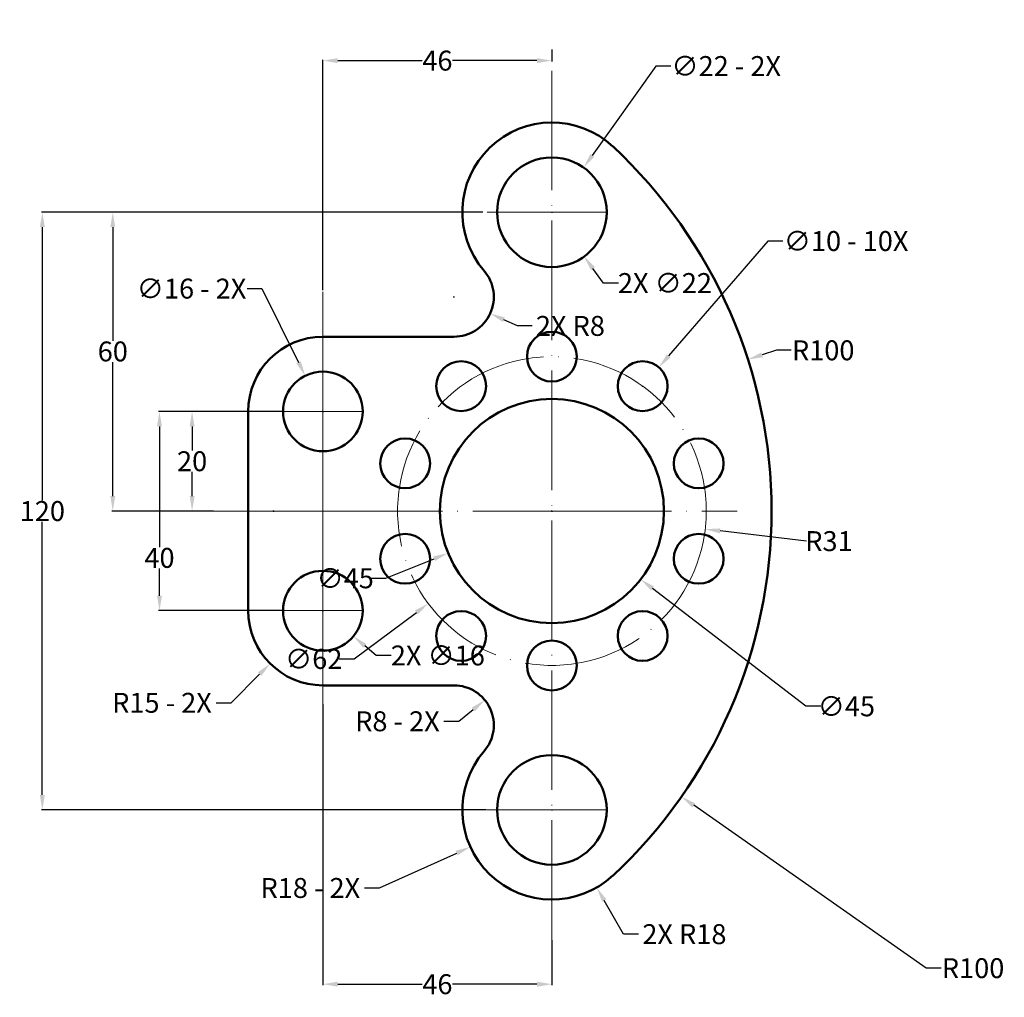
# Model space of a CAD drawing. Units: inches. Extents: x 498 to 696, y 198 to 394.
import ezdxf

# ---------------------------------------------------------------- set-up
doc = ezdxf.new("R2010")
doc.units = ezdxf.units.IN
doc.header["$MEASUREMENT"] = 0
doc.linetypes.add('ACAD_ISO04W100', pattern=[30, 24, -3, 0, -3])
for name, color, linetype, lineweight in [('M-CNTR', 4, 'ACAD_ISO04W100', 18), ('M-DIMS', 2, 'Continuous', 25), ('M-OUTL', 7, 'Continuous', 50)]:
    doc.layers.add(name, color=color, linetype=linetype, lineweight=lineweight)
doc.styles.get("Standard").update_dxf_attribs({"font": 'arial.ttf'})
doc.dimstyles.get("Standard").update_dxf_attribs({"dimtxt": 4, "dimasz": 3, "dimexe": 0.18, "dimexo": 0.0625, "dimgap": 0.09, "dimtad": 0, "dimtih": 1, "dimtoh": 1, "dimdec": 0, "dimzin": 0, "dimdsep": 46, "dimtxsty": 'Standard', "dimcen": 0.09, "dimclrd": 1, "dimclre": 1, "dimadec": 0, "dimazin": 0, "dimtfac": 1, "dimtdec": 0, "dimtofl": 0, "dimtmove": 0, "dimatfit": 3, "dimfxl": 1, "dimtolj": 1, "dimtzin": 0, "dimarcsym": 0})

# ---------------------------------------------------------------- blocks, each defined once
blk = doc.blocks.new('*U1')
blk.add_circle((0, 0), 5)
blk = doc.blocks.new('*U2')
at = {"layer": 'M-OUTL', "color": 0, "linetype": 'ByBlock', "lineweight": -2, "transparency": 16777216}
blk.add_blockref('*U1', (604.82, 326.53), dxfattribs=at)
for p, rotation in [((586.6, 320.6), 35.99999999999999), ((623.04, 320.6), 324), ((575.34, 305.1), 72), ((634.3, 305.1), 288), ((575.34, 285.95), 108), ((634.3, 285.95), 252), ((586.6, 270.45), 144), ((623.04, 270.45), 216), ((604.82, 264.53), 180)]:
    blk.add_blockref('*U1', p, dxfattribs=dict(at, rotation=rotation))
blk = doc.blocks.new('*D3')
at = {"layer": 'Defpoints', "color": 0, "transparency": 16777216}
for p in [(591.02, 355.53), (502.47, 235.53), (591.74, 235.53)]:
    blk.add_point(p, dxfattribs=at)
at = {"layer": 'M-DIMS', "color": 0, "lineweight": -2, "transparency": 16777216}
for p, q in [((590.96, 355.53), (502.29, 355.53)), ((502.47, 352.53), (502.47, 297.66)), ((502.47, 238.53), (502.47, 293.39)), ((591.68, 235.53), (502.29, 235.53))]:
    blk.add_line(p, q, dxfattribs=at)
at = {"layer": 'M-DIMS', "color": 0, "transparency": 16777216}
for points in [[(501.97, 352.53), (502.97, 352.53), (502.47, 355.53)], [(501.97, 238.53), (502.97, 238.53), (502.47, 235.53)]]:
    blk.add_solid(points, dxfattribs=at)
at = {"layer": 'M-DIMS', "color": 0, "transparency": 16777216, "insert": (502.47, 295.53), "char_height": 4, "attachment_point": 5}
blk.add_mtext('\\A1;120', dxfattribs=at)
blk = doc.blocks.new('*D4')
at = {"layer": 'Defpoints', "color": 0, "transparency": 16777216}
for p in [(591.02, 355.53), (516.62, 295.53), (536.94, 295.53)]:
    blk.add_point(p, dxfattribs=at)
at = {"layer": 'M-DIMS', "color": 0, "lineweight": -2, "transparency": 16777216}
for p, q in [((590.96, 355.53), (516.44, 355.53)), ((516.62, 352.53), (516.62, 329.7)), ((516.62, 298.53), (516.62, 325.44)), ((536.88, 295.53), (516.44, 295.53))]:
    blk.add_line(p, q, dxfattribs=at)
at = {"layer": 'M-DIMS', "color": 0, "transparency": 16777216}
for points in [[(516.12, 352.53), (517.12, 352.53), (516.62, 355.53)], [(516.12, 298.53), (517.12, 298.53), (516.62, 295.53)]]:
    blk.add_solid(points, dxfattribs=at)
at = {"layer": 'M-DIMS', "color": 0, "transparency": 16777216, "insert": (516.62, 327.57), "char_height": 4, "attachment_point": 5}
blk.add_mtext('\\A1;60', dxfattribs=at)
blk = doc.blocks.new('*D5')
at = {"layer": 'Defpoints', "color": 0, "transparency": 16777216}
for p in [(555.26, 322.69), (562.38, 308.36)]:
    blk.add_point(p, dxfattribs=at)
at = {"layer": 'M-DIMS', "color": 0, "lineweight": -2, "transparency": 16777216}
for p, q in [((543.58, 340.19), (546.58, 340.19)), ((546.58, 340.19), (553.93, 325.38)), ((558.73, 315.53), (558.91, 315.53)), ((558.82, 315.44), (558.82, 315.62))]:
    blk.add_line(p, q, dxfattribs=at)
at = {"layer": 'M-DIMS', "color": 0, "transparency": 16777216}
blk.add_solid([(554.38, 325.6), (553.48, 325.16), (555.26, 322.69)], dxfattribs=at)
at = {"layer": 'M-DIMS', "color": 0, "transparency": 16777216, "insert": (532.44, 340.19), "char_height": 4, "attachment_point": 5}
blk.add_mtext('\\A1;∅16 - 2X', dxfattribs=at)
blk = doc.blocks.new('*D6')
at = {"layer": 'Defpoints', "color": 0, "transparency": 16777216}
for p in [(550.82, 315.53), (532.55, 295.53), (536.94, 295.53)]:
    blk.add_point(p, dxfattribs=at)
at = {"layer": 'M-DIMS', "color": 0, "lineweight": -2, "transparency": 16777216}
for p, q in [((550.76, 315.53), (532.37, 315.53)), ((532.55, 312.53), (532.55, 307.66)), ((532.55, 298.53), (532.55, 303.39)), ((536.88, 295.53), (532.37, 295.53))]:
    blk.add_line(p, q, dxfattribs=at)
at = {"layer": 'M-DIMS', "color": 0, "transparency": 16777216}
for points in [[(532.05, 312.53), (533.05, 312.53), (532.55, 315.53)], [(532.05, 298.53), (533.05, 298.53), (532.55, 295.53)]]:
    blk.add_solid(points, dxfattribs=at)
at = {"layer": 'M-DIMS', "color": 0, "transparency": 16777216, "insert": (532.55, 305.53), "char_height": 4, "attachment_point": 5}
blk.add_mtext('\\A1;20', dxfattribs=at)
blk = doc.blocks.new('*D7')
at = {"layer": 'Defpoints', "color": 0, "transparency": 16777216}
for p in [(550.82, 315.53), (526, 275.53), (550.82, 275.53)]:
    blk.add_point(p, dxfattribs=at)
at = {"layer": 'M-DIMS', "color": 0, "lineweight": -2, "transparency": 16777216}
for p, q in [((550.76, 315.53), (525.82, 315.53)), ((526, 312.53), (526, 288.25)), ((526, 278.53), (526, 283.99)), ((550.76, 275.53), (525.82, 275.53))]:
    blk.add_line(p, q, dxfattribs=at)
at = {"layer": 'M-DIMS', "color": 0, "transparency": 16777216}
for points in [[(525.5, 312.53), (526.5, 312.53), (526, 315.53)], [(525.5, 278.53), (526.5, 278.53), (526, 275.53)]]:
    blk.add_solid(points, dxfattribs=at)
at = {"layer": 'M-DIMS', "color": 0, "transparency": 16777216, "insert": (526, 286.12), "char_height": 4, "attachment_point": 5}
blk.add_mtext('\\A1;40', dxfattribs=at)
blk = doc.blocks.new('*D8')
at = {"layer": 'Defpoints', "color": 0, "transparency": 16777216}
for p in [(558.82, 275.53), (548.23, 264.9)]:
    blk.add_point(p, dxfattribs=at)
at = {"layer": 'M-DIMS', "color": 0, "lineweight": -2, "transparency": 16777216}
for p, q in [((558.73, 275.53), (558.91, 275.53)), ((558.82, 275.44), (558.82, 275.62)), ((540.38, 257.03), (546.11, 262.78)), ((537.38, 257.03), (540.38, 257.03))]:
    blk.add_line(p, q, dxfattribs=at)
at = {"layer": 'M-DIMS', "color": 0, "transparency": 16777216}
blk.add_solid([(545.76, 263.13), (546.46, 262.43), (548.23, 264.9)], dxfattribs=at)
at = {"layer": 'M-DIMS', "color": 0, "transparency": 16777216, "insert": (526.5, 257.03), "char_height": 4, "attachment_point": 5}
blk.add_mtext('\\A1;R15 - 2X', dxfattribs=at)
blk = doc.blocks.new('*D9')
at = {"layer": 'Defpoints', "color": 0, "transparency": 16777216}
for p in [(591.35, 257.58), (585.15, 252.53)]:
    blk.add_point(p, dxfattribs=at)
at = {"layer": 'M-DIMS', "color": 0, "lineweight": -2, "transparency": 16777216}
for p, q in [((586.12, 253.32), (589.02, 255.69)), ((583.12, 253.32), (586.12, 253.32))]:
    blk.add_line(p, q, dxfattribs=at)
at = {"layer": 'M-DIMS', "color": 0, "transparency": 16777216}
blk.add_solid([(588.71, 256.07), (589.34, 255.3), (591.35, 257.58)], dxfattribs=at)
at = {"layer": 'M-DIMS', "color": 0, "transparency": 16777216, "insert": (573.79, 253.32), "char_height": 4, "attachment_point": 5}
blk.add_mtext('\\A1;R8 - 2X', dxfattribs=at)
blk = doc.blocks.new('*D10')
at = {"layer": 'Defpoints', "color": 0, "transparency": 16777216}
for p in [(604.82, 235.53), (588.42, 228.1)]:
    blk.add_point(p, dxfattribs=at)
at = {"layer": 'M-DIMS', "color": 0, "lineweight": -2, "transparency": 16777216}
for p, q in [((604.73, 235.53), (604.91, 235.53)), ((604.82, 235.44), (604.82, 235.62)), ((570.18, 219.85), (585.69, 226.87)), ((567.18, 219.85), (570.18, 219.85))]:
    blk.add_line(p, q, dxfattribs=at)
at = {"layer": 'M-DIMS', "color": 0, "transparency": 16777216}
blk.add_solid([(585.48, 227.32), (585.9, 226.41), (588.42, 228.1)], dxfattribs=at)
at = {"layer": 'M-DIMS', "color": 0, "transparency": 16777216, "insert": (556.3, 219.85), "char_height": 4, "attachment_point": 5}
blk.add_mtext('\\A1;R18 - 2X', dxfattribs=at)
blk = doc.blocks.new('*D11')
at = {"layer": 'Defpoints', "color": 0, "transparency": 16777216}
for p in [(558.82, 256.82), (604.82, 209.44), (604.82, 200.53)]:
    blk.add_point(p, dxfattribs=at)
at = {"layer": 'M-DIMS', "color": 0, "lineweight": -2, "transparency": 16777216}
for p, q in [((558.82, 256.75), (558.82, 200.35)), ((604.82, 209.37), (604.82, 200.35)), ((561.82, 200.53), (578.79, 200.53)), ((601.82, 200.53), (584.85, 200.53))]:
    blk.add_line(p, q, dxfattribs=at)
at = {"layer": 'M-DIMS', "color": 0, "transparency": 16777216}
for points in [[(561.82, 201.03), (561.82, 200.03), (558.82, 200.53)], [(601.82, 201.03), (601.82, 200.03), (604.82, 200.53)]]:
    blk.add_solid(points, dxfattribs=at)
at = {"layer": 'M-DIMS', "color": 0, "transparency": 16777216, "insert": (581.82, 200.53), "char_height": 4, "attachment_point": 5}
blk.add_mtext('\\A1;46', dxfattribs=at)
blk = doc.blocks.new('*D12')
at = {"layer": 'Defpoints', "color": 0, "transparency": 16777216}
for p in [(586.98, 309.24), (622.66, 281.81)]:
    blk.add_point(p, dxfattribs=at)
at = {"layer": 'M-DIMS', "color": 0, "lineweight": -2, "transparency": 16777216}
for p, q in [((604.73, 295.53), (604.91, 295.53)), ((604.82, 295.44), (604.82, 295.62)), ((655.81, 256.32), (625.04, 279.98)), ((658.81, 256.32), (655.81, 256.32))]:
    blk.add_line(p, q, dxfattribs=at)
at = {"layer": 'M-DIMS', "color": 0, "transparency": 16777216}
blk.add_solid([(625.34, 280.38), (624.73, 279.59), (622.66, 281.81)], dxfattribs=at)
at = {"layer": 'M-DIMS', "color": 0, "transparency": 16777216, "insert": (663.96, 256.32), "char_height": 4, "attachment_point": 5}
blk.add_mtext('\\A1;∅45', dxfattribs=at)
blk = doc.blocks.new('*D13')
at = {"layer": 'Defpoints', "color": 0, "transparency": 16777216}
for p in [(604.82, 295.53), (635.61, 291.89)]:
    blk.add_point(p, dxfattribs=at)
at = {"layer": 'M-DIMS', "color": 0, "lineweight": -2, "transparency": 16777216}
for p, q in [((604.73, 295.53), (604.91, 295.53)), ((604.82, 295.44), (604.82, 295.62)), ((655.98, 289.49), (638.59, 291.54))]:
    blk.add_line(p, q, dxfattribs=at)
at = {"layer": 'M-DIMS', "color": 0, "transparency": 16777216}
blk.add_solid([(638.64, 292.04), (638.53, 291.04), (635.61, 291.89)], dxfattribs=at)
at = {"layer": 'M-DIMS', "color": 0, "transparency": 16777216, "insert": (660.46, 289.49), "char_height": 4, "attachment_point": 5}
blk.add_mtext('\\A1;R31', dxfattribs=at)
blk = doc.blocks.new('*D14')
at = {"layer": 'Defpoints', "color": 0, "transparency": 16777216}
for p in [(644.18, 325.97), (548.93, 295.53)]:
    blk.add_point(p, dxfattribs=at)
at = {"layer": 'M-DIMS', "color": 0, "lineweight": -2, "transparency": 16777216}
for p, q in [((649.9, 327.8), (647.04, 326.89)), ((652.9, 327.8), (649.9, 327.8)), ((548.84, 295.53), (549.02, 295.53)), ((548.93, 295.44), (548.93, 295.62))]:
    blk.add_line(p, q, dxfattribs=at)
at = {"layer": 'M-DIMS', "color": 0, "transparency": 16777216}
blk.add_solid([(646.89, 327.36), (647.19, 326.41), (644.18, 325.97)], dxfattribs=at)
at = {"layer": 'M-DIMS', "color": 0, "transparency": 16777216, "insert": (659.31, 327.8), "char_height": 4, "attachment_point": 5}
blk.add_mtext('\\A1;R100', dxfattribs=at)
blk = doc.blocks.new('*D15')
at = {"layer": 'Defpoints', "color": 0, "transparency": 16777216}
for p in [(626.31, 324.39), (619.77, 316.82)]:
    blk.add_point(p, dxfattribs=at)
at = {"layer": 'M-DIMS', "color": 0, "lineweight": -2, "transparency": 16777216}
for p, q in [((648.21, 349.74), (628.27, 326.66)), ((651.21, 349.74), (648.21, 349.74)), ((622.95, 320.6), (623.13, 320.6)), ((623.04, 320.51), (623.04, 320.69))]:
    blk.add_line(p, q, dxfattribs=at)
at = {"layer": 'M-DIMS', "color": 0, "transparency": 16777216}
blk.add_solid([(627.89, 326.99), (628.65, 326.33), (626.31, 324.39)], dxfattribs=at)
at = {"layer": 'M-DIMS', "color": 0, "transparency": 16777216, "insert": (663.91, 349.74), "char_height": 4, "attachment_point": 5}
blk.add_mtext('\\A1;∅10 - 10X', dxfattribs=at)
blk = doc.blocks.new('*D16')
at = {"layer": 'Defpoints', "color": 0, "transparency": 16777216}
for p in [(611.2, 364.49), (598.45, 346.56)]:
    blk.add_point(p, dxfattribs=at)
at = {"layer": 'M-DIMS', "color": 0, "lineweight": -2, "transparency": 16777216}
for p, q in [((625.69, 384.87), (612.93, 366.93)), ((628.69, 384.87), (625.69, 384.87)), ((604.73, 355.53), (604.91, 355.53)), ((604.82, 355.44), (604.82, 355.62))]:
    blk.add_line(p, q, dxfattribs=at)
at = {"layer": 'M-DIMS', "color": 0, "transparency": 16777216}
blk.add_solid([(612.53, 367.22), (613.34, 366.64), (611.2, 364.49)], dxfattribs=at)
at = {"layer": 'M-DIMS', "color": 0, "transparency": 16777216, "insert": (639.83, 384.87), "char_height": 4, "attachment_point": 5}
blk.add_mtext('\\A1;∅22 - 2X', dxfattribs=at)
blk = doc.blocks.new('*D17')
at = {"layer": 'Defpoints', "color": 0, "transparency": 16777216}
for p in [(604.82, 388.24), (604.82, 385.96), (558.82, 339.8)]:
    blk.add_point(p, dxfattribs=at)
at = {"layer": 'M-DIMS', "color": 0, "lineweight": -2, "transparency": 16777216}
for p, q in [((604.82, 388.17), (604.82, 385.78)), ((558.82, 339.86), (558.82, 386.14)), ((561.82, 385.96), (578.79, 385.96)), ((601.82, 385.96), (584.85, 385.96))]:
    blk.add_line(p, q, dxfattribs=at)
at = {"layer": 'M-DIMS', "color": 0, "transparency": 16777216}
for points in [[(561.82, 386.46), (561.82, 385.46), (558.82, 385.96)], [(601.82, 386.46), (601.82, 385.46), (604.82, 385.96)]]:
    blk.add_solid(points, dxfattribs=at)
at = {"layer": 'M-DIMS', "color": 0, "transparency": 16777216, "insert": (581.82, 385.96), "char_height": 4, "attachment_point": 5}
blk.add_mtext('\\A1;46', dxfattribs=at)
blk = doc.blocks.new('HOLE-MOUNT-D16')
blk.add_circle((8, 8), 8)
blk = doc.blocks.new('HOLE-EAR-D22')
blk.add_circle((11, 11), 11)
blk = doc.blocks.new('*D20')
at = {"layer": 'Defpoints', "color": 0, "transparency": 16777216}
for p in [(548.93, 295.53), (630.84, 238.17)]:
    blk.add_point(p, dxfattribs=at)
at = {"layer": 'M-DIMS', "color": 1, "lineweight": -2, "transparency": 16777216}
for p, q in [((548.84, 295.53), (549.02, 295.53)), ((548.93, 295.44), (548.93, 295.62)), ((679.99, 203.75), (633.3, 236.45)), ((682.99, 203.75), (679.99, 203.75))]:
    blk.add_line(p, q, dxfattribs=at)
at = {"layer": 'M-DIMS', "color": 1, "transparency": 16777216}
blk.add_solid([(633.59, 236.86), (633.01, 236.04), (630.84, 238.17)], dxfattribs=at)
at = {"layer": 'M-DIMS', "color": 0, "transparency": 16777216, "insert": (689.41, 203.75), "char_height": 4, "attachment_point": 5}
blk.add_mtext('\\A1;R100', dxfattribs=at)
blk = doc.blocks.new('*D21')
at = {"layer": 'Defpoints', "color": 0, "transparency": 16777216}
for p in [(625.68, 303.96), (583.96, 287.09)]:
    blk.add_point(p, dxfattribs=at)
at = {"layer": 'M-DIMS', "color": 1, "lineweight": -2, "transparency": 16777216}
for p, q in [((604.73, 295.53), (604.91, 295.53)), ((604.82, 295.44), (604.82, 295.62)), ((571.45, 282.02), (581.18, 285.96)), ((568.45, 282.02), (571.45, 282.02))]:
    blk.add_line(p, q, dxfattribs=at)
at = {"layer": 'M-DIMS', "color": 1, "transparency": 16777216}
blk.add_solid([(580.99, 286.42), (581.37, 285.5), (583.96, 287.09)], dxfattribs=at)
at = {"layer": 'M-DIMS', "color": 0, "transparency": 16777216, "insert": (563.3, 282.02), "char_height": 4, "attachment_point": 5}
blk.add_mtext('\\A1;∅45', dxfattribs=at)
blk = doc.blocks.new('*D22')
at = {"layer": 'Defpoints', "color": 0, "transparency": 16777216}
for p in [(629.65, 314.09), (579.99, 276.96)]:
    blk.add_point(p, dxfattribs=at)
at = {"layer": 'M-DIMS', "color": 1, "lineweight": -2, "transparency": 16777216}
for p, q in [((604.73, 295.53), (604.91, 295.53)), ((604.82, 295.44), (604.82, 295.62)), ((565.09, 265.83), (577.59, 275.17)), ((562.09, 265.83), (565.09, 265.83))]:
    blk.add_line(p, q, dxfattribs=at)
at = {"layer": 'M-DIMS', "color": 1, "transparency": 16777216}
blk.add_solid([(577.29, 275.57), (577.89, 274.77), (579.99, 276.96)], dxfattribs=at)
at = {"layer": 'M-DIMS', "color": 0, "transparency": 16777216, "insert": (556.98, 265.83), "char_height": 4, "attachment_point": 5}
blk.add_mtext('\\A1;∅62', dxfattribs=at)
blk = doc.blocks.new('*D23')
at = {"layer": 'Defpoints', "color": 0, "transparency": 16777216}
for p in [(604.82, 235.53), (613.82, 219.94)]:
    blk.add_point(p, dxfattribs=at)
at = {"layer": 'M-DIMS', "color": 1, "lineweight": -2, "transparency": 16777216}
for p, q in [((604.73, 235.53), (604.91, 235.53)), ((604.82, 235.44), (604.82, 235.62)), ((619.22, 210.58), (615.32, 217.34)), ((622.22, 210.58), (619.22, 210.58))]:
    blk.add_line(p, q, dxfattribs=at)
at = {"layer": 'M-DIMS', "color": 1, "transparency": 16777216}
blk.add_solid([(615.75, 217.59), (614.89, 217.09), (613.82, 219.94)], dxfattribs=at)
at = {"layer": 'M-DIMS', "color": 0, "transparency": 16777216, "insert": (631.43, 210.58), "char_height": 4, "attachment_point": 5}
blk.add_mtext('\\A1;2X R18', dxfattribs=at)
blk = doc.blocks.new('*D24')
at = {"layer": 'Defpoints', "color": 0, "transparency": 16777216}
for p in [(585.15, 338.53), (592.42, 335.2)]:
    blk.add_point(p, dxfattribs=at)
at = {"layer": 'M-DIMS', "color": 1, "lineweight": -2, "transparency": 16777216}
for p, q in [((585.06, 338.53), (585.24, 338.53)), ((585.15, 338.44), (585.15, 338.62)), ((597.88, 332.7), (595.15, 333.95)), ((600.88, 332.7), (597.88, 332.7))]:
    blk.add_line(p, q, dxfattribs=at)
at = {"layer": 'M-DIMS', "color": 1, "transparency": 16777216}
blk.add_solid([(595.36, 334.4), (594.94, 333.49), (592.42, 335.2)], dxfattribs=at)
at = {"layer": 'M-DIMS', "color": 0, "transparency": 16777216, "insert": (608.53, 332.7), "char_height": 4, "attachment_point": 5}
blk.add_mtext('\\A1;2X R8', dxfattribs=at)
blk = doc.blocks.new('*D25')
at = {"layer": 'Defpoints', "color": 0, "transparency": 16777216}
for p in [(598.34, 364.42), (611.3, 346.63)]:
    blk.add_point(p, dxfattribs=at)
at = {"layer": 'M-DIMS', "color": 1, "lineweight": -2, "transparency": 16777216}
for p, q in [((604.73, 355.53), (604.91, 355.53)), ((604.82, 355.44), (604.82, 355.62)), ((615.18, 341.3), (613.06, 344.21)), ((618.18, 341.3), (615.18, 341.3))]:
    blk.add_line(p, q, dxfattribs=at)
at = {"layer": 'M-DIMS', "color": 1, "transparency": 16777216}
blk.add_solid([(613.47, 344.5), (612.66, 343.91), (611.3, 346.63)], dxfattribs=at)
at = {"layer": 'M-DIMS', "color": 0, "transparency": 16777216, "insert": (627.52, 341.3), "char_height": 4, "attachment_point": 5}
blk.add_mtext('\\A1;2X ∅22', dxfattribs=at)
blk = doc.blocks.new('*D26')
at = {"layer": 'Defpoints', "color": 0, "transparency": 16777216}
for p in [(552.69, 280.66), (564.95, 270.39)]:
    blk.add_point(p, dxfattribs=at)
at = {"layer": 'M-DIMS', "color": 1, "lineweight": -2, "transparency": 16777216}
for p, q in [((558.73, 275.53), (558.91, 275.53)), ((558.82, 275.44), (558.82, 275.62)), ((569.55, 266.53), (567.25, 268.46)), ((572.55, 266.53), (569.55, 266.53))]:
    blk.add_line(p, q, dxfattribs=at)
at = {"layer": 'M-DIMS', "color": 1, "transparency": 16777216}
blk.add_solid([(567.57, 268.84), (566.93, 268.08), (564.95, 270.39)], dxfattribs=at)
at = {"layer": 'M-DIMS', "color": 0, "transparency": 16777216, "insert": (581.91, 266.53), "char_height": 4, "attachment_point": 5}
blk.add_mtext('\\A1;2X ∅16', dxfattribs=at)

msp = doc.modelspace()

# ---------------------------------------------------------------- linework, layer by layer
at = {"layer": 'M-CNTR'}
for p, q in [((604.82, 209.44), (604.82, 388.24)), ((615.82, 355.53), (591.02, 355.53)), ((566.82, 315.53), (550.82, 315.53)), ((566.82, 275.53), (550.82, 275.53)), ((615.82, 235.53), (591.74, 235.53))]:
    msp.add_line(p, q, dxfattribs=at)
for points in [[(558.82, 256.82), (558.82, 275.53), (558.82, 295.53), (558.82, 315.53), (558.82, 339.8)], [(536.94, 295.53), (558.82, 295.53), (604.82, 295.53), (642, 295.53)]]:
    msp.add_lwpolyline(points, dxfattribs=at)
msp.add_circle((604.82, 295.53), 31, dxfattribs=at)
at = {"layer": 'M-OUTL'}
for p, q in [((558.82, 330.53), (585.15, 330.53)), ((543.82, 315.53), (543.82, 275.53)), ((558.82, 260.53), (585.15, 260.53))]:
    msp.add_line(p, q, dxfattribs=at)
msp.add_circle((604.82, 295.53), 22.5, dxfattribs=at)
for centre, radius, start, end in [((604.82, 355.53), 18, 47.0297, 220.8322), ((548.93, 295.53), 100, 312.9703, 47.0297), ((585.15, 338.53), 8, 270, 40.8322), ((558.82, 315.53), 15, 90, 180), ((558.82, 275.53), 15, 180, 270), ((585.15, 252.53), 8, 319.1678, 90), ((604.82, 235.53), 18, 139.1678, 312.9703)]:
    msp.add_arc(centre, radius, start, end, dxfattribs=at)

# ---------------------------------------------------------------- block references
for name, p in [('HOLE-EAR-D22', (593.82, 344.52)), ('*U2', (0, 0)), ('HOLE-MOUNT-D16', (550.82, 307.52)), ('HOLE-MOUNT-D16', (550.82, 267.52)), ('HOLE-EAR-D22', (593.82, 224.53))]:
    msp.add_blockref(name, p, dxfattribs=at)

# ---------------------------------------------------------------- dimensions: what is measured, and where the dimension line sits
at = {"layer": 'M-DIMS'}
for p1, p2, text, override, picture, middle in [((598.45, 346.56), (611.2, 364.49), '<> - 2X', {"dimclrd": 0, "dimclre": 0, "dimclrt": 0}, '*D16', (639.83, 384.87)), ((598.34, 364.42), (611.3, 346.63), '2X <>', {"dimdec": 0, "dimlfac": 1, "dimrnd": 0, "dimzin": 0, "dimdsep": 46, "dimlunit": 2}, '*D25', (627.52, 341.3)), ((619.77, 316.82), (626.31, 324.39), '<> - 10X', {"dimclrd": 0, "dimclre": 0, "dimclrt": 0}, '*D15', (663.91, 349.74)), ((562.38, 308.36), (555.26, 322.69), '<> - 2X', {"dimclrd": 0, "dimclre": 0, "dimclrt": 0}, '*D5', (532.44, 340.19)), ((552.69, 280.66), (564.95, 270.39), '2X <>', {"dimdec": 0, "dimlfac": 1, "dimrnd": 0, "dimzin": 0, "dimdsep": 46, "dimlunit": 2}, '*D26', (581.91, 266.53))]:
    dim = msp.add_diameter_dim_2p(p1=p1, p2=p2, text=text, dimstyle='Standard', override=override, dxfattribs=at)
    dim.commit()
    dim.dimension.update_dxf_attribs({"geometry": picture, "text_midpoint": middle, "dimtype": 163})
for base, p1, p2, picture, middle in [((604.82, 385.96), (558.82, 339.8), (604.82, 388.24), '*D17', (581.82, 385.96)), ((604.82, 200.53), (558.82, 256.82), (604.82, 209.44), '*D11', (581.82, 200.53))]:
    dim = msp.add_linear_dim(base=base, p1=p1, p2=p2, dimstyle='Standard', override={"dimclrd": 0, "dimclre": 0, "dimclrt": 0}, dxfattribs=at)
    dim.commit()
    dim.dimension.update_dxf_attribs({"geometry": picture, "text_midpoint": middle})
for base, p1, p2, picture, middle in [((502.47, 235.53), (591.02, 355.53), (591.74, 235.53), '*D3', (502.47, 295.53)), ((532.55, 295.53), (550.82, 315.53), (536.94, 295.53), '*D6', (532.55, 305.53))]:
    dim = msp.add_linear_dim(base=base, p1=p1, p2=p2, angle=90, dimstyle='Standard', override={"dimclrd": 0, "dimclre": 0, "dimclrt": 0}, dxfattribs=at)
    dim.commit()
    dim.dimension.update_dxf_attribs({"geometry": picture, "text_midpoint": middle})
for base, p1, p2, picture, middle in [((516.62, 295.53), (591.02, 355.53), (536.94, 295.53), '*D4', (516.62, 327.57)), ((526, 275.53), (550.82, 315.53), (550.82, 275.53), '*D7', (526, 286.12))]:
    dim = msp.add_linear_dim(base=base, p1=p1, p2=p2, angle=90, dimstyle='Standard', override={"dimclrd": 0, "dimclre": 0, "dimclrt": 0}, dxfattribs=at)
    dim.commit()
    dim.dimension.update_dxf_attribs({"geometry": picture, "text_midpoint": middle, "dimtype": 160})
dim = msp.add_radius_dim(center=(585.15, 338.53), mpoint=(592.42, 335.2), text='2X <>', dimstyle='Standard', override={"dimdec": 0, "dimlfac": 1, "dimrnd": 0, "dimzin": 0, "dimdsep": 46, "dimlunit": 2}, dxfattribs=at)
dim.commit()
dim.dimension.update_dxf_attribs({"geometry": '*D24', "text_midpoint": (608.53, 332.7)})
dim = msp.add_radius_dim(center=(548.93, 295.53), mpoint=(644.18, 325.97), dimstyle='Standard', override={"dimclrd": 0, "dimclre": 0, "dimclrt": 0}, dxfattribs=at)
dim.commit()
dim.dimension.update_dxf_attribs({"geometry": '*D14', "text_midpoint": (659.31, 327.8)})
for p1, p2, override, picture, middle in [((629.65, 314.09), (579.99, 276.96), {"dimdec": 0, "dimlfac": 1, "dimrnd": 0, "dimzin": 0, "dimdsep": 46, "dimlunit": 2}, '*D22', (556.98, 265.83)), ((586.98, 309.24), (622.66, 281.81), {"dimclrd": 0, "dimclre": 0, "dimclrt": 0}, '*D12', (663.96, 256.32)), ((625.68, 303.96), (583.96, 287.09), {"dimdec": 0, "dimlfac": 1, "dimrnd": 0, "dimzin": 0, "dimdsep": 46, "dimlunit": 2}, '*D21', (563.3, 282.02))]:
    dim = msp.add_diameter_dim_2p(p1=p1, p2=p2, dimstyle='Standard', override=override, dxfattribs=at)
    dim.commit()
    dim.dimension.update_dxf_attribs({"geometry": picture, "text_midpoint": middle, "dimtype": 163})
for center, mpoint, override, picture, middle in [((548.93, 295.53), (630.84, 238.17), {"dimdec": 0, "dimlfac": 1, "dimrnd": 0, "dimzin": 0, "dimdsep": 46, "dimlunit": 2}, '*D20', (689.41, 203.75)), ((604.82, 295.53), (635.61, 291.89), {"dimclrd": 0, "dimclre": 0, "dimclrt": 0}, '*D13', (655.98, 289.49))]:
    dim = msp.add_radius_dim(center=center, mpoint=mpoint, dimstyle='Standard', override=override, dxfattribs=at)
    dim.commit()
    dim.dimension.update_dxf_attribs({"geometry": picture, "text_midpoint": middle, "dimtype": 164})
for center, mpoint, text, override, picture, middle in [((558.82, 275.53), (548.23, 264.9), '<> - 2X', {"dimclrd": 0, "dimclre": 0, "dimclrt": 0}, '*D8', (526.5, 257.03)), ((585.15, 252.53), (591.35, 257.58), '<> - 2X', {"dimclrd": 0, "dimclre": 0, "dimclrt": 0}, '*D9', (573.79, 253.32)), ((604.82, 235.53), (588.42, 228.1), '<> - 2X', {"dimclrd": 0, "dimclre": 0, "dimclrt": 0}, '*D10', (556.3, 219.85)), ((604.82, 235.53), (613.82, 219.94), '2X <>', {"dimdec": 0, "dimlfac": 1, "dimrnd": 0, "dimzin": 0, "dimdsep": 46, "dimlunit": 2}, '*D23', (631.43, 210.58))]:
    dim = msp.add_radius_dim(center=center, mpoint=mpoint, text=text, dimstyle='Standard', override=override, dxfattribs=at)
    dim.commit()
    dim.dimension.update_dxf_attribs({"geometry": picture, "text_midpoint": middle, "dimtype": 164})

doc.saveas('drawing.dxf')
